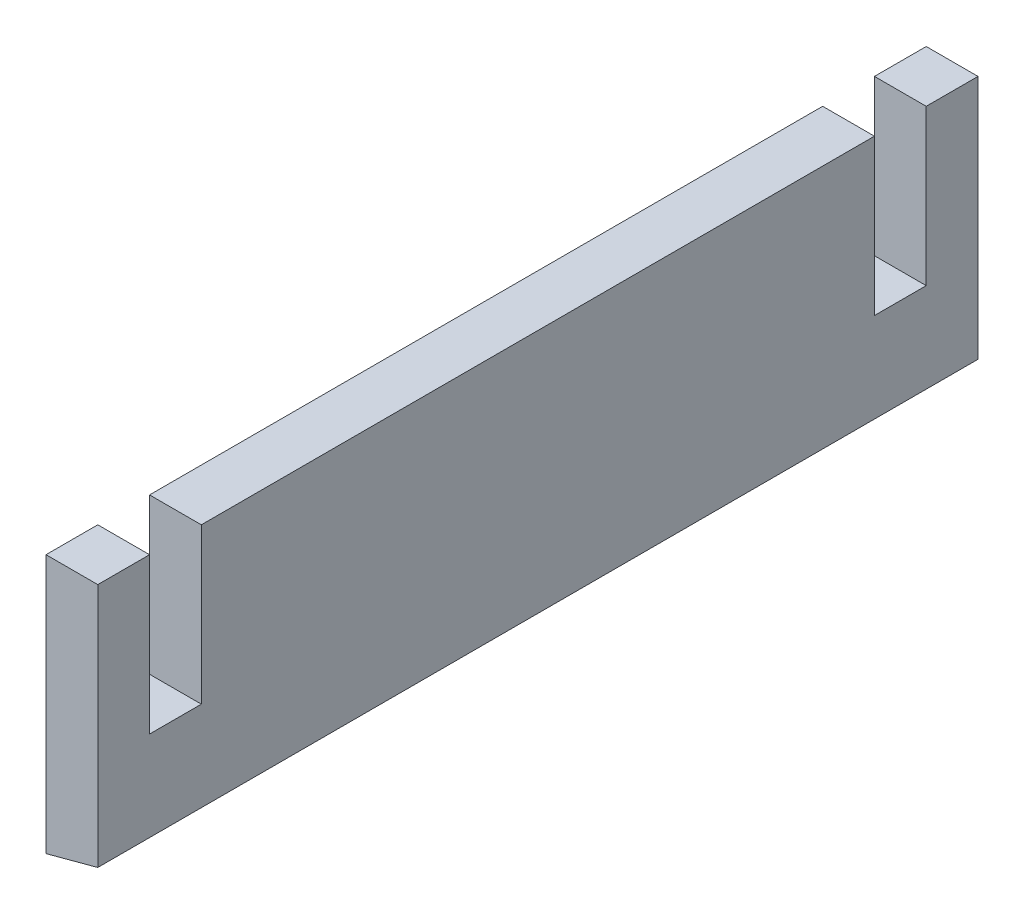
ISO-10303-21;
HEADER;
FILE_DESCRIPTION(('STEP AP214'),'2;1');
FILE_NAME('part.step','',(''),(''),'','','');
FILE_SCHEMA(('AUTOMOTIVE_DESIGN { 1 0 10303 214 1 1 1 1 }'));
ENDSEC;
DATA;
#1=APPLICATION_CONTEXT('core data for automotive mechanical design processes');
#2=APPLICATION_PROTOCOL_DEFINITION('international standard','automotive_design',2000,#1);
#3=PRODUCT_CONTEXT('',#1,'mechanical');
#4=PRODUCT('Part','Part','',(#3));
#5=PRODUCT_RELATED_PRODUCT_CATEGORY('part','',(#4));
#6=PRODUCT_DEFINITION_FORMATION('','',#4);
#7=PRODUCT_DEFINITION_CONTEXT('part definition',#1,'design');
#8=PRODUCT_DEFINITION('design','',#6,#7);
#9=PRODUCT_DEFINITION_SHAPE('','',#8);
#10=(LENGTH_UNIT() NAMED_UNIT(*) SI_UNIT(.MILLI.,.METRE.));
#11=(NAMED_UNIT(*) PLANE_ANGLE_UNIT() SI_UNIT($,.RADIAN.));
#12=(NAMED_UNIT(*) SI_UNIT($,.STERADIAN.) SOLID_ANGLE_UNIT());
#13=UNCERTAINTY_MEASURE_WITH_UNIT(LENGTH_MEASURE(1.E-05),#10,'distance_accuracy_value','');
#14=(GEOMETRIC_REPRESENTATION_CONTEXT(3) GLOBAL_UNCERTAINTY_ASSIGNED_CONTEXT((#13)) GLOBAL_UNIT_ASSIGNED_CONTEXT((#10,
#11,#12)) REPRESENTATION_CONTEXT('',''));
#15=CARTESIAN_POINT('',(0.,0.,0.));
#16=DIRECTION('',(0.,0.,1.));
#17=DIRECTION('',(1.,0.,0.));
#18=AXIS2_PLACEMENT_3D('',#15,#16,#17);
#19=CARTESIAN_POINT('',(5.,50.,0.));
#20=DIRECTION('',(0.,0.,-1.));
#21=DIRECTION('',(0.,1.,0.));
#22=AXIS2_PLACEMENT_3D('',#19,#20,#21);
#23=PLANE('',#22);
#24=DIRECTION('',(0.,-1.,0.));
#25=VECTOR('',#24,1.);
#26=CARTESIAN_POINT('',(-5.,50.,0.));
#27=LINE('',#26,#25);
#28=CARTESIAN_POINT('',(-5.,50.,0.));
#29=VERTEX_POINT('',#28);
#30=CARTESIAN_POINT('',(-5.,0.,0.));
#31=VERTEX_POINT('',#30);
#32=EDGE_CURVE('E157',#29,#31,#27,.T.);
#33=ORIENTED_EDGE('',*,*,#32,.T.);
#34=DIRECTION('',(0.965925826289068,0.258819045102521,0.));
#35=VECTOR('',#34,1.);
#36=CARTESIAN_POINT('',(-5.,0.,0.));
#37=LINE('',#36,#35);
#38=CARTESIAN_POINT('',(5.,2.67949192431124,0.));
#39=VERTEX_POINT('',#38);
#40=EDGE_CURVE('E11',#39,#31,#37,.F.);
#41=ORIENTED_EDGE('',*,*,#40,.F.);
#42=DIRECTION('',(0.,-1.,0.));
#43=VECTOR('',#42,1.);
#44=CARTESIAN_POINT('',(5.,50.,0.));
#45=LINE('',#44,#43);
#46=CARTESIAN_POINT('',(5.,50.,0.));
#47=VERTEX_POINT('',#46);
#48=EDGE_CURVE('E181',#47,#39,#45,.T.);
#49=ORIENTED_EDGE('',*,*,#48,.F.);
#50=DIRECTION('',(-1.,0.,0.));
#51=VECTOR('',#50,1.);
#52=CARTESIAN_POINT('',(5.,50.,0.));
#53=LINE('',#52,#51);
#54=EDGE_CURVE('E154',#47,#29,#53,.T.);
#55=ORIENTED_EDGE('',*,*,#54,.T.);
#56=EDGE_LOOP('',(#33,#41,#49,#55));
#57=FACE_BOUND('',#56,.T.);
#58=ADVANCED_FACE('F39',(#57),#23,.F.);
#59=CARTESIAN_POINT('',(-5.,0.,0.));
#60=DIRECTION('',(0.258819045102521,-0.965925826289068,0.));
#61=DIRECTION('',(0.965925826289068,0.258819045102521,0.));
#62=AXIS2_PLACEMENT_3D('',#59,#60,#61);
#63=PLANE('',#62);
#64=DIRECTION('',(0.,0.,-1.));
#65=VECTOR('',#64,1.);
#66=CARTESIAN_POINT('',(-5.,0.,0.));
#67=LINE('',#66,#65);
#68=CARTESIAN_POINT('',(-5.,0.,-170.));
#69=VERTEX_POINT('',#68);
#70=EDGE_CURVE('E165',#31,#69,#67,.T.);
#71=ORIENTED_EDGE('',*,*,#70,.T.);
#72=DIRECTION('',(0.965925826289068,0.258819045102521,0.));
#73=VECTOR('',#72,1.);
#74=CARTESIAN_POINT('',(4.33012701892219,2.50000000000001,-170.));
#75=LINE('',#74,#73);
#76=CARTESIAN_POINT('',(5.,2.67949192431123,-170.));
#77=VERTEX_POINT('',#76);
#78=EDGE_CURVE('E43',#77,#69,#75,.F.);
#79=ORIENTED_EDGE('',*,*,#78,.F.);
#80=DIRECTION('',(0.,0.,1.));
#81=VECTOR('',#80,1.);
#82=CARTESIAN_POINT('',(5.,2.67949192431123,0.));
#83=LINE('',#82,#81);
#84=EDGE_CURVE('E103',#39,#77,#83,.F.);
#85=ORIENTED_EDGE('',*,*,#84,.F.);
#86=ORIENTED_EDGE('',*,*,#40,.T.);
#87=EDGE_LOOP('',(#71,#79,#85,#86));
#88=FACE_BOUND('',#87,.T.);
#89=ADVANCED_FACE('F41',(#88),#63,.T.);
#90=CARTESIAN_POINT('',(5.,0.,-170.));
#91=DIRECTION('',(0.,0.,1.));
#92=DIRECTION('',(1.,0.,0.));
#93=AXIS2_PLACEMENT_3D('',#90,#91,#92);
#94=PLANE('',#93);
#95=DIRECTION('',(0.,1.,0.));
#96=VECTOR('',#95,1.);
#97=CARTESIAN_POINT('',(-5.,0.,-170.));
#98=LINE('',#97,#96);
#99=CARTESIAN_POINT('',(-5.,50.,-170.));
#100=VERTEX_POINT('',#99);
#101=EDGE_CURVE('E163',#69,#100,#98,.T.);
#102=ORIENTED_EDGE('',*,*,#101,.T.);
#103=DIRECTION('',(-1.,0.,0.));
#104=VECTOR('',#103,1.);
#105=CARTESIAN_POINT('',(5.,50.,-170.));
#106=LINE('',#105,#104);
#107=CARTESIAN_POINT('',(5.,50.,-170.));
#108=VERTEX_POINT('',#107);
#109=EDGE_CURVE('E201',#108,#100,#106,.T.);
#110=ORIENTED_EDGE('',*,*,#109,.F.);
#111=DIRECTION('',(0.,1.,0.));
#112=VECTOR('',#111,1.);
#113=CARTESIAN_POINT('',(5.,0.,-170.));
#114=LINE('',#113,#112);
#115=EDGE_CURVE('E109',#77,#108,#114,.T.);
#116=ORIENTED_EDGE('',*,*,#115,.F.);
#117=ORIENTED_EDGE('',*,*,#78,.T.);
#118=EDGE_LOOP('',(#102,#110,#116,#117));
#119=FACE_BOUND('',#118,.T.);
#120=ADVANCED_FACE('F239',(#119),#94,.F.);
#121=CARTESIAN_POINT('',(5.,50.,-170.));
#122=DIRECTION('',(0.,-1.,0.));
#123=DIRECTION('',(0.,0.,-1.));
#124=AXIS2_PLACEMENT_3D('',#121,#122,#123);
#125=PLANE('',#124);
#126=DIRECTION('',(0.,0.,1.));
#127=VECTOR('',#126,1.);
#128=CARTESIAN_POINT('',(-5.,50.,-170.));
#129=LINE('',#128,#127);
#130=CARTESIAN_POINT('',(-5.,50.,-160.));
#131=VERTEX_POINT('',#130);
#132=EDGE_CURVE('E167',#100,#131,#129,.T.);
#133=ORIENTED_EDGE('',*,*,#132,.T.);
#134=DIRECTION('',(-1.,0.,0.));
#135=VECTOR('',#134,1.);
#136=CARTESIAN_POINT('',(5.,50.,-160.));
#137=LINE('',#136,#135);
#138=CARTESIAN_POINT('',(5.,50.,-160.));
#139=VERTEX_POINT('',#138);
#140=EDGE_CURVE('E199',#139,#131,#137,.T.);
#141=ORIENTED_EDGE('',*,*,#140,.F.);
#142=DIRECTION('',(0.,0.,1.));
#143=VECTOR('',#142,1.);
#144=CARTESIAN_POINT('',(5.,50.,-170.));
#145=LINE('',#144,#143);
#146=EDGE_CURVE('E202',#108,#139,#145,.T.);
#147=ORIENTED_EDGE('',*,*,#146,.F.);
#148=ORIENTED_EDGE('',*,*,#109,.T.);
#149=EDGE_LOOP('',(#133,#141,#147,#148));
#150=FACE_BOUND('',#149,.T.);
#151=ADVANCED_FACE('F242',(#150),#125,.F.);
#152=CARTESIAN_POINT('',(5.,50.,-160.));
#153=DIRECTION('',(0.,0.,-1.));
#154=DIRECTION('',(-1.,0.,0.));
#155=AXIS2_PLACEMENT_3D('',#152,#153,#154);
#156=PLANE('',#155);
#157=DIRECTION('',(0.,-1.,0.));
#158=VECTOR('',#157,1.);
#159=CARTESIAN_POINT('',(-5.,50.,-160.));
#160=LINE('',#159,#158);
#161=CARTESIAN_POINT('',(-5.,20.,-160.));
#162=VERTEX_POINT('',#161);
#163=EDGE_CURVE('E169',#131,#162,#160,.T.);
#164=ORIENTED_EDGE('',*,*,#163,.T.);
#165=DIRECTION('',(-1.,0.,0.));
#166=VECTOR('',#165,1.);
#167=CARTESIAN_POINT('',(5.,20.,-160.));
#168=LINE('',#167,#166);
#169=CARTESIAN_POINT('',(5.,20.,-160.));
#170=VERTEX_POINT('',#169);
#171=EDGE_CURVE('E197',#170,#162,#168,.T.);
#172=ORIENTED_EDGE('',*,*,#171,.F.);
#173=DIRECTION('',(0.,-1.,0.));
#174=VECTOR('',#173,1.);
#175=CARTESIAN_POINT('',(5.,50.,-160.));
#176=LINE('',#175,#174);
#177=EDGE_CURVE('E215',#139,#170,#176,.T.);
#178=ORIENTED_EDGE('',*,*,#177,.F.);
#179=ORIENTED_EDGE('',*,*,#140,.T.);
#180=EDGE_LOOP('',(#164,#172,#178,#179));
#181=FACE_BOUND('',#180,.T.);
#182=ADVANCED_FACE('F246',(#181),#156,.F.);
#183=CARTESIAN_POINT('',(5.,20.,-160.));
#184=DIRECTION('',(0.,-1.,0.));
#185=DIRECTION('',(0.,0.,-1.));
#186=AXIS2_PLACEMENT_3D('',#183,#184,#185);
#187=PLANE('',#186);
#188=DIRECTION('',(0.,0.,1.));
#189=VECTOR('',#188,1.);
#190=CARTESIAN_POINT('',(-5.,20.,-160.));
#191=LINE('',#190,#189);
#192=CARTESIAN_POINT('',(-5.,20.,-150.));
#193=VERTEX_POINT('',#192);
#194=EDGE_CURVE('E168',#162,#193,#191,.T.);
#195=ORIENTED_EDGE('',*,*,#194,.T.);
#196=DIRECTION('',(-1.,0.,0.));
#197=VECTOR('',#196,1.);
#198=CARTESIAN_POINT('',(5.,20.,-150.));
#199=LINE('',#198,#197);
#200=CARTESIAN_POINT('',(5.,20.,-150.));
#201=VERTEX_POINT('',#200);
#202=EDGE_CURVE('E191',#201,#193,#199,.T.);
#203=ORIENTED_EDGE('',*,*,#202,.F.);
#204=DIRECTION('',(0.,0.,1.));
#205=VECTOR('',#204,1.);
#206=CARTESIAN_POINT('',(5.,20.,-160.));
#207=LINE('',#206,#205);
#208=EDGE_CURVE('E212',#170,#201,#207,.T.);
#209=ORIENTED_EDGE('',*,*,#208,.F.);
#210=ORIENTED_EDGE('',*,*,#171,.T.);
#211=EDGE_LOOP('',(#195,#203,#209,#210));
#212=FACE_BOUND('',#211,.T.);
#213=ADVANCED_FACE('F255',(#212),#187,.F.);
#214=CARTESIAN_POINT('',(5.,20.,-150.));
#215=DIRECTION('',(0.,0.,1.));
#216=DIRECTION('',(0.,-1.,0.));
#217=AXIS2_PLACEMENT_3D('',#214,#215,#216);
#218=PLANE('',#217);
#219=DIRECTION('',(0.,1.,0.));
#220=VECTOR('',#219,1.);
#221=CARTESIAN_POINT('',(-5.,20.,-150.));
#222=LINE('',#221,#220);
#223=CARTESIAN_POINT('',(-5.,50.,-150.));
#224=VERTEX_POINT('',#223);
#225=EDGE_CURVE('E171',#193,#224,#222,.T.);
#226=ORIENTED_EDGE('',*,*,#225,.T.);
#227=DIRECTION('',(-1.,0.,0.));
#228=VECTOR('',#227,1.);
#229=CARTESIAN_POINT('',(5.,50.,-150.));
#230=LINE('',#229,#228);
#231=CARTESIAN_POINT('',(5.,50.,-150.));
#232=VERTEX_POINT('',#231);
#233=EDGE_CURVE('E192',#232,#224,#230,.T.);
#234=ORIENTED_EDGE('',*,*,#233,.F.);
#235=DIRECTION('',(0.,1.,0.));
#236=VECTOR('',#235,1.);
#237=CARTESIAN_POINT('',(5.,20.,-150.));
#238=LINE('',#237,#236);
#239=EDGE_CURVE('E216',#201,#232,#238,.T.);
#240=ORIENTED_EDGE('',*,*,#239,.F.);
#241=ORIENTED_EDGE('',*,*,#202,.T.);
#242=EDGE_LOOP('',(#226,#234,#240,#241));
#243=FACE_BOUND('',#242,.T.);
#244=ADVANCED_FACE('F260',(#243),#218,.F.);
#245=CARTESIAN_POINT('',(5.,50.,-150.));
#246=DIRECTION('',(0.,-1.,0.));
#247=DIRECTION('',(0.,0.,-1.));
#248=AXIS2_PLACEMENT_3D('',#245,#246,#247);
#249=PLANE('',#248);
#250=DIRECTION('',(0.,0.,1.));
#251=VECTOR('',#250,1.);
#252=CARTESIAN_POINT('',(-5.,50.,-150.));
#253=LINE('',#252,#251);
#254=CARTESIAN_POINT('',(-5.,50.,-20.));
#255=VERTEX_POINT('',#254);
#256=EDGE_CURVE('E173',#224,#255,#253,.T.);
#257=ORIENTED_EDGE('',*,*,#256,.T.);
#258=DIRECTION('',(-1.,0.,0.));
#259=VECTOR('',#258,1.);
#260=CARTESIAN_POINT('',(5.,50.,-20.));
#261=LINE('',#260,#259);
#262=CARTESIAN_POINT('',(5.,50.,-20.));
#263=VERTEX_POINT('',#262);
#264=EDGE_CURVE('E190',#263,#255,#261,.T.);
#265=ORIENTED_EDGE('',*,*,#264,.F.);
#266=DIRECTION('',(0.,0.,1.));
#267=VECTOR('',#266,1.);
#268=CARTESIAN_POINT('',(5.,50.,-150.));
#269=LINE('',#268,#267);
#270=EDGE_CURVE('E217',#232,#263,#269,.T.);
#271=ORIENTED_EDGE('',*,*,#270,.F.);
#272=ORIENTED_EDGE('',*,*,#233,.T.);
#273=EDGE_LOOP('',(#257,#265,#271,#272));
#274=FACE_BOUND('',#273,.T.);
#275=ADVANCED_FACE('F221',(#274),#249,.F.);
#276=CARTESIAN_POINT('',(5.,50.,-20.));
#277=DIRECTION('',(0.,0.,-1.));
#278=DIRECTION('',(0.,1.,0.));
#279=AXIS2_PLACEMENT_3D('',#276,#277,#278);
#280=PLANE('',#279);
#281=DIRECTION('',(0.,-1.,0.));
#282=VECTOR('',#281,1.);
#283=CARTESIAN_POINT('',(-5.,50.,-20.));
#284=LINE('',#283,#282);
#285=CARTESIAN_POINT('',(-5.,20.,-20.));
#286=VERTEX_POINT('',#285);
#287=EDGE_CURVE('E177',#255,#286,#284,.T.);
#288=ORIENTED_EDGE('',*,*,#287,.T.);
#289=DIRECTION('',(-1.,0.,0.));
#290=VECTOR('',#289,1.);
#291=CARTESIAN_POINT('',(5.,20.,-20.));
#292=LINE('',#291,#290);
#293=CARTESIAN_POINT('',(5.,20.,-20.));
#294=VERTEX_POINT('',#293);
#295=EDGE_CURVE('E149',#294,#286,#292,.T.);
#296=ORIENTED_EDGE('',*,*,#295,.F.);
#297=DIRECTION('',(0.,-1.,0.));
#298=VECTOR('',#297,1.);
#299=CARTESIAN_POINT('',(5.,50.,-20.));
#300=LINE('',#299,#298);
#301=EDGE_CURVE('E140',#263,#294,#300,.T.);
#302=ORIENTED_EDGE('',*,*,#301,.F.);
#303=ORIENTED_EDGE('',*,*,#264,.T.);
#304=EDGE_LOOP('',(#288,#296,#302,#303));
#305=FACE_BOUND('',#304,.T.);
#306=ADVANCED_FACE('F230',(#305),#280,.F.);
#307=CARTESIAN_POINT('',(5.,20.,-20.));
#308=DIRECTION('',(0.,-1.,0.));
#309=DIRECTION('',(0.,0.,-1.));
#310=AXIS2_PLACEMENT_3D('',#307,#308,#309);
#311=PLANE('',#310);
#312=DIRECTION('',(0.,0.,1.));
#313=VECTOR('',#312,1.);
#314=CARTESIAN_POINT('',(-5.,20.,-20.));
#315=LINE('',#314,#313);
#316=CARTESIAN_POINT('',(-5.,20.,-10.));
#317=VERTEX_POINT('',#316);
#318=EDGE_CURVE('E148',#286,#317,#315,.T.);
#319=ORIENTED_EDGE('',*,*,#318,.T.);
#320=DIRECTION('',(-1.,0.,0.));
#321=VECTOR('',#320,1.);
#322=CARTESIAN_POINT('',(5.,20.,-10.));
#323=LINE('',#322,#321);
#324=CARTESIAN_POINT('',(5.,20.,-10.));
#325=VERTEX_POINT('',#324);
#326=EDGE_CURVE('E141',#325,#317,#323,.T.);
#327=ORIENTED_EDGE('',*,*,#326,.F.);
#328=DIRECTION('',(0.,0.,1.));
#329=VECTOR('',#328,1.);
#330=CARTESIAN_POINT('',(5.,20.,-20.));
#331=LINE('',#330,#329);
#332=EDGE_CURVE('E128',#294,#325,#331,.T.);
#333=ORIENTED_EDGE('',*,*,#332,.F.);
#334=ORIENTED_EDGE('',*,*,#295,.T.);
#335=EDGE_LOOP('',(#319,#327,#333,#334));
#336=FACE_BOUND('',#335,.T.);
#337=ADVANCED_FACE('F145',(#336),#311,.F.);
#338=CARTESIAN_POINT('',(5.,20.,-10.));
#339=DIRECTION('',(0.,0.,1.));
#340=DIRECTION('',(1.,0.,0.));
#341=AXIS2_PLACEMENT_3D('',#338,#339,#340);
#342=PLANE('',#341);
#343=DIRECTION('',(0.,1.,0.));
#344=VECTOR('',#343,1.);
#345=CARTESIAN_POINT('',(-5.,20.,-10.));
#346=LINE('',#345,#344);
#347=CARTESIAN_POINT('',(-5.,50.,-10.));
#348=VERTEX_POINT('',#347);
#349=EDGE_CURVE('E176',#317,#348,#346,.T.);
#350=ORIENTED_EDGE('',*,*,#349,.T.);
#351=DIRECTION('',(-1.,0.,0.));
#352=VECTOR('',#351,1.);
#353=CARTESIAN_POINT('',(5.,50.,-10.));
#354=LINE('',#353,#352);
#355=CARTESIAN_POINT('',(5.,50.,-10.));
#356=VERTEX_POINT('',#355);
#357=EDGE_CURVE('E147',#356,#348,#354,.T.);
#358=ORIENTED_EDGE('',*,*,#357,.F.);
#359=DIRECTION('',(0.,1.,0.));
#360=VECTOR('',#359,1.);
#361=CARTESIAN_POINT('',(5.,20.,-10.));
#362=LINE('',#361,#360);
#363=EDGE_CURVE('E133',#325,#356,#362,.T.);
#364=ORIENTED_EDGE('',*,*,#363,.F.);
#365=ORIENTED_EDGE('',*,*,#326,.T.);
#366=EDGE_LOOP('',(#350,#358,#364,#365));
#367=FACE_BOUND('',#366,.T.);
#368=ADVANCED_FACE('F155',(#367),#342,.F.);
#369=CARTESIAN_POINT('',(5.,50.,-10.));
#370=DIRECTION('',(0.,-1.,0.));
#371=DIRECTION('',(0.,0.,-1.));
#372=AXIS2_PLACEMENT_3D('',#369,#370,#371);
#373=PLANE('',#372);
#374=DIRECTION('',(0.,0.,1.));
#375=VECTOR('',#374,1.);
#376=CARTESIAN_POINT('',(-5.,50.,-10.));
#377=LINE('',#376,#375);
#378=EDGE_CURVE('E182',#348,#29,#377,.T.);
#379=ORIENTED_EDGE('',*,*,#378,.T.);
#380=ORIENTED_EDGE('',*,*,#54,.F.);
#381=DIRECTION('',(0.,0.,1.));
#382=VECTOR('',#381,1.);
#383=CARTESIAN_POINT('',(5.,50.,-10.));
#384=LINE('',#383,#382);
#385=EDGE_CURVE('E60',#356,#47,#384,.T.);
#386=ORIENTED_EDGE('',*,*,#385,.F.);
#387=ORIENTED_EDGE('',*,*,#357,.T.);
#388=EDGE_LOOP('',(#379,#380,#386,#387));
#389=FACE_BOUND('',#388,.T.);
#390=ADVANCED_FACE('F231',(#389),#373,.F.);
#391=CARTESIAN_POINT('',(5.,0.,0.));
#392=DIRECTION('',(1.,0.,0.));
#393=DIRECTION('',(0.,0.,-1.));
#394=AXIS2_PLACEMENT_3D('',#391,#392,#393);
#395=PLANE('',#394);
#396=ORIENTED_EDGE('',*,*,#48,.T.);
#397=ORIENTED_EDGE('',*,*,#84,.T.);
#398=ORIENTED_EDGE('',*,*,#115,.T.);
#399=ORIENTED_EDGE('',*,*,#146,.T.);
#400=ORIENTED_EDGE('',*,*,#177,.T.);
#401=ORIENTED_EDGE('',*,*,#208,.T.);
#402=ORIENTED_EDGE('',*,*,#239,.T.);
#403=ORIENTED_EDGE('',*,*,#270,.T.);
#404=ORIENTED_EDGE('',*,*,#301,.T.);
#405=ORIENTED_EDGE('',*,*,#332,.T.);
#406=ORIENTED_EDGE('',*,*,#363,.T.);
#407=ORIENTED_EDGE('',*,*,#385,.T.);
#408=EDGE_LOOP('',(#396,#397,#398,#399,#400,#401,#402,#403,#404,#405,#406,#407));
#409=FACE_BOUND('',#408,.T.);
#410=ADVANCED_FACE('F131',(#409),#395,.T.);
#411=CARTESIAN_POINT('',(-5.,0.,0.));
#412=DIRECTION('',(1.,0.,0.));
#413=DIRECTION('',(0.,0.,-1.));
#414=AXIS2_PLACEMENT_3D('',#411,#412,#413);
#415=PLANE('',#414);
#416=ORIENTED_EDGE('',*,*,#32,.F.);
#417=ORIENTED_EDGE('',*,*,#378,.F.);
#418=ORIENTED_EDGE('',*,*,#349,.F.);
#419=ORIENTED_EDGE('',*,*,#318,.F.);
#420=ORIENTED_EDGE('',*,*,#287,.F.);
#421=ORIENTED_EDGE('',*,*,#256,.F.);
#422=ORIENTED_EDGE('',*,*,#225,.F.);
#423=ORIENTED_EDGE('',*,*,#194,.F.);
#424=ORIENTED_EDGE('',*,*,#163,.F.);
#425=ORIENTED_EDGE('',*,*,#132,.F.);
#426=ORIENTED_EDGE('',*,*,#101,.F.);
#427=ORIENTED_EDGE('',*,*,#70,.F.);
#428=EDGE_LOOP('',(#416,#417,#418,#419,#420,#421,#422,#423,#424,#425,#426,#427));
#429=FACE_BOUND('',#428,.T.);
#430=ADVANCED_FACE('F232',(#429),#415,.F.);
#431=CLOSED_SHELL('',(#58,#89,#120,#151,#182,#213,#244,#275,#306,#337,#368,#390,#410,#430));
#432=MANIFOLD_SOLID_BREP('B2',#431);
#433=ADVANCED_BREP_SHAPE_REPRESENTATION('',(#18,#432),#14);
#434=SHAPE_DEFINITION_REPRESENTATION(#9,#433);
ENDSEC;
END-ISO-10303-21;
